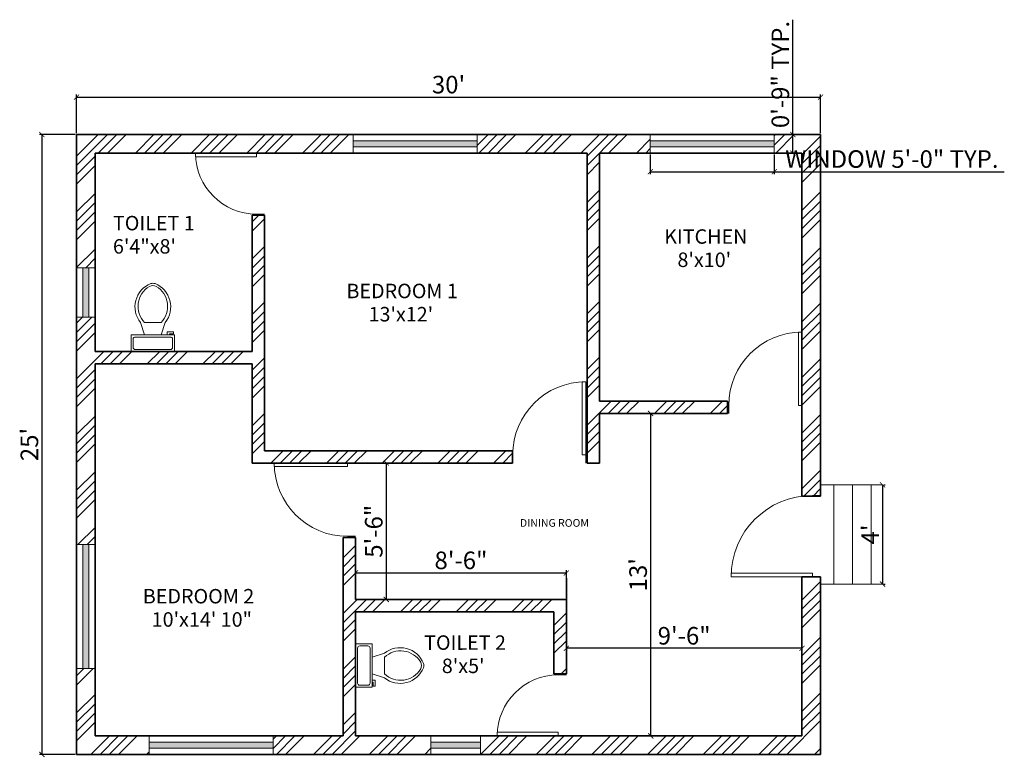
# Model space of a CAD drawing. Units: inches. Extents: x 3799 to 20199, y 1682 to 8087.
# Tile 24 of 30: x 16056 to 16532, y 2726 to 3083. Entities that reach past the tile are written whole.
import ezdxf

# ---------------------------------------------------------------- set-up
doc = ezdxf.new("R2010")
doc.units = ezdxf.units.IN
for name, color, linetype, lineweight in [('A-ANNO-DIMS', 2, 'Continuous', 18), ('A-AREA-IDEN', 7, 'Continuous', 18), ('A-DOOR', 3, 'Continuous', 18), ('A-FLOR-FIXT', 9, 'Continuous', 18), ('A-FLOR-STRS', 41, 'Continuous', 18), ('A-GLAZ', 152, 'Continuous', 18), ('A-GLAZ-PATT', 152, 'Continuous', 13), ('A-WALL', 7, 'Continuous', 35), ('A-WALL-PATT', 252, 'Continuous', 13)]:
    doc.layers.add(name, color=color, linetype=linetype, lineweight=lineweight)
doc.styles.get("Standard").update_dxf_attribs({"font": 'arial.ttf'})
doc.dimstyles.new('ISO-25', dxfattribs={"dimtxt": 8.5, "dimasz": 2.5, "dimexe": 1.25, "dimexo": 0.625, "dimtad": 1, "dimdec": 0, "dimlunit": 3, "dimtxsty": 'Standard', "dimblk": 'ARCHTICK', "dimcen": 2.5, "dimadec": 0, "dimazin": 0, "dimtfac": 1, "dimtdec": 0, "dimtmove": 0, "dimatfit": 3, "dimfxl": 1, "dimarcsym": 0})

# ---------------------------------------------------------------- blocks, each defined once
blk = doc.blocks.new('*U123')
for p, q in [((0, 0), (0, -100)), ((-900, 0), (-900, -100))]:
    blk.add_line(p, q)
blk.add_lwpolyline([(0, 0), (0, 900), (-43.75, 900), (-43.75, 0)], close=True)
blk.add_arc((0, 0), 900, 90, 180)
blk = doc.blocks.new('*U48')
for p, q in [((-750, 0), (-750, -100)), ((0, 0), (0, -100))]:
    blk.add_line(p, q)
blk.add_lwpolyline([(0, 0), (0, 750), (-43.75, 750), (-43.75, 0)], close=True)
blk.add_arc((0, 0), 750, 90, 180)
blk = doc.blocks.new('*U124')
for p, q in [((0, 0), (0, -100)), ((-900, 0), (-900, -100))]:
    blk.add_line(p, q)
blk.add_lwpolyline([(0, 0), (0, 900), (-43.75, 900), (-43.75, 0)], close=True)
blk.add_arc((0, 0), 900, 90, 180)
blk = doc.blocks.new('*U125')
for p, q in [((0, 0), (0, -100)), ((750, 0), (750, -100))]:
    blk.add_line(p, q)
blk.add_lwpolyline([(0, 0), (0, 750), (43.75, 750), (43.75, 0)], close=True)
blk.add_arc((0, 0), 750, 0, 90)
blk = doc.blocks.new('*U126')
for p, q in [((0, 0), (0, -100)), ((1000, 0), (1000, -100))]:
    blk.add_line(p, q)
blk.add_lwpolyline([(0, 0), (0, 1000), (43.75, 1000), (43.75, 0)], close=True)
blk.add_arc((0, 0), 1000, 0, 90)
blk = doc.blocks.new('_ArchTick')
at = {"color": 0, "linetype": 'ByBlock', "const_width": 0.15}
blk.add_lwpolyline([(-0.5, -0.5), (0.5, 0.5)], dxfattribs=at)
blk = doc.blocks.new('*D127')
at = {"layer": 'A-ANNO-DIMS', "color": 0, "lineweight": -2, "transparency": 16777216}
for p, q in [((16473.58, 2858.27), (16473.58, 2810.27)), ((16474.21, 2858.27), (16474.83, 2858.27)), ((16474.21, 2810.27), (16474.83, 2810.27))]:
    blk.add_line(p, q, dxfattribs=at)
at = {"layer": 'Defpoints', "color": 0, "transparency": 16777216}
for p in [(16473.58, 2858.27), (16473.58, 2810.27), (16473.58, 2810.27)]:
    blk.add_point(p, dxfattribs=at)
at = {"layer": 'A-ANNO-DIMS', "color": 0, "lineweight": -2, "transparency": 16777216, "xscale": 2.5, "yscale": 2.5, "zscale": 2.5}
for p, rotation in [((16473.58, 2858.27), 90), ((16473.58, 2810.27), 270)]:
    blk.add_blockref('_ArchTick', p, dxfattribs=dict(at, rotation=rotation))
at = {"layer": 'A-ANNO-DIMS', "color": 0, "transparency": 16777216, "insert": (16468.71, 2834.27), "char_height": 8.5, "attachment_point": 5, "rotation": 90}
blk.add_mtext("4'", dxfattribs=at)
blk = doc.blocks.new('*D128')
at = {"layer": 'A-ANNO-DIMS', "color": 0, "lineweight": -2, "transparency": 16777216}
for p, q in [((16293.96, 2868.83), (16232.22, 2868.83)), ((16233.47, 2868.83), (16233.47, 2802.83)), ((16293.96, 2802.83), (16232.22, 2802.83))]:
    blk.add_line(p, q, dxfattribs=at)
at = {"layer": 'Defpoints', "color": 0, "transparency": 16777216}
for p in [(16294.58, 2868.83), (16233.47, 2802.83), (16294.58, 2802.83)]:
    blk.add_point(p, dxfattribs=at)
at = {"layer": 'A-ANNO-DIMS', "color": 0, "lineweight": -2, "transparency": 16777216, "xscale": 2.5, "yscale": 2.5, "zscale": 2.5}
for p, rotation in [((16233.47, 2868.83), 90), ((16233.47, 2802.83), 270)]:
    blk.add_blockref('_ArchTick', p, dxfattribs=dict(at, rotation=rotation))
at = {"layer": 'A-ANNO-DIMS', "color": 0, "transparency": 16777216, "insert": (16228.5, 2835.83), "char_height": 8.5, "attachment_point": 5, "rotation": 90}
blk.add_mtext('5\'-6"', dxfattribs=at)
blk = doc.blocks.new('*D129')
at = {"layer": 'A-ANNO-DIMS', "color": 0, "lineweight": -2, "transparency": 16777216}
for p, q in [((16218.58, 2803.46), (16218.58, 2816.94)), ((16218.58, 2815.69), (16320.58, 2815.69)), ((16320.58, 2803.46), (16320.58, 2816.94))]:
    blk.add_line(p, q, dxfattribs=at)
at = {"layer": 'Defpoints', "color": 0, "transparency": 16777216}
for p in [(16320.58, 2815.69), (16218.58, 2802.83), (16320.58, 2802.83)]:
    blk.add_point(p, dxfattribs=at)
at = {"layer": 'A-ANNO-DIMS', "color": 0, "lineweight": -2, "transparency": 16777216, "xscale": 2.5, "yscale": 2.5, "zscale": 2.5, "rotation": 180}
blk.add_blockref('_ArchTick', (16218.58, 2815.69), dxfattribs=at)
at = {"layer": 'A-ANNO-DIMS', "color": 0, "lineweight": -2, "transparency": 16777216, "xscale": 2.5, "yscale": 2.5, "zscale": 2.5}
blk.add_blockref('_ArchTick', (16320.58, 2815.69), dxfattribs=at)
at = {"layer": 'A-ANNO-DIMS', "color": 0, "transparency": 16777216, "insert": (16269.58, 2820.66), "char_height": 8.5, "attachment_point": 5}
blk.add_mtext('8\'-6"', dxfattribs=at)
blk = doc.blocks.new('*D130')
at = {"layer": 'A-ANNO-DIMS', "color": 0, "lineweight": -2, "transparency": 16777216}
for p, q in [((16337.21, 2892.83), (16362.62, 2892.83)), ((16361.37, 2892.83), (16361.37, 2736.83)), ((16337.21, 2736.83), (16362.62, 2736.83))]:
    blk.add_line(p, q, dxfattribs=at)
at = {"layer": 'Defpoints', "color": 0, "transparency": 16777216}
for p in [(16336.58, 2892.83), (16336.58, 2736.83), (16361.37, 2736.83)]:
    blk.add_point(p, dxfattribs=at)
at = {"layer": 'A-ANNO-DIMS', "color": 0, "lineweight": -2, "transparency": 16777216, "xscale": 2.5, "yscale": 2.5, "zscale": 2.5}
for p, rotation in [((16361.37, 2892.83), 90), ((16361.37, 2736.83), 270)]:
    blk.add_blockref('_ArchTick', p, dxfattribs=dict(at, rotation=rotation))
at = {"layer": 'A-ANNO-DIMS', "color": 0, "transparency": 16777216, "insert": (16356.4, 2814.83), "char_height": 8.5, "attachment_point": 5, "rotation": 90}
blk.add_mtext("13'", dxfattribs=at)
blk = doc.blocks.new('*D131')
at = {"layer": 'A-ANNO-DIMS', "color": 0, "lineweight": -2, "transparency": 16777216}
for p, q in [((16320.58, 2813.18), (16320.58, 2777.94)), ((16434.58, 2813.18), (16434.58, 2777.94)), ((16434.58, 2779.19), (16320.58, 2779.19))]:
    blk.add_line(p, q, dxfattribs=at)
at = {"layer": 'Defpoints', "color": 0, "transparency": 16777216}
for p in [(16320.58, 2813.8), (16434.58, 2813.8), (16320.58, 2779.19)]:
    blk.add_point(p, dxfattribs=at)
at = {"layer": 'A-ANNO-DIMS', "color": 0, "lineweight": -2, "transparency": 16777216, "xscale": 2.5, "yscale": 2.5, "zscale": 2.5, "rotation": 180}
blk.add_blockref('_ArchTick', (16320.58, 2779.19), dxfattribs=at)
at = {"layer": 'A-ANNO-DIMS', "color": 0, "lineweight": -2, "transparency": 16777216, "xscale": 2.5, "yscale": 2.5, "zscale": 2.5}
blk.add_blockref('_ArchTick', (16434.58, 2779.19), dxfattribs=at)
at = {"layer": 'A-ANNO-DIMS', "color": 0, "transparency": 16777216, "insert": (16377.58, 2784.16), "char_height": 8.5, "attachment_point": 5}
blk.add_mtext('9\'-6"', dxfattribs=at)
blk = doc.blocks.new('*D132')
at = {"layer": 'A-ANNO-DIMS', "color": 0, "lineweight": -2, "transparency": 16777216}
for p, q in [((16083.58, 3028.46), (16083.58, 3047.16)), ((16083.58, 3045.91), (16443.58, 3045.91)), ((16443.58, 3028.46), (16443.58, 3047.16))]:
    blk.add_line(p, q, dxfattribs=at)
at = {"layer": 'Defpoints', "color": 0, "transparency": 16777216}
for p in [(16443.58, 3045.91), (16083.58, 3027.83), (16443.58, 3027.83)]:
    blk.add_point(p, dxfattribs=at)
at = {"layer": 'A-ANNO-DIMS', "color": 0, "lineweight": -2, "transparency": 16777216, "xscale": 2.5, "yscale": 2.5, "zscale": 2.5, "rotation": 180}
blk.add_blockref('_ArchTick', (16083.58, 3045.91), dxfattribs=at)
at = {"layer": 'A-ANNO-DIMS', "color": 0, "lineweight": -2, "transparency": 16777216, "xscale": 2.5, "yscale": 2.5, "zscale": 2.5}
blk.add_blockref('_ArchTick', (16443.58, 3045.91), dxfattribs=at)
at = {"layer": 'A-ANNO-DIMS', "color": 0, "transparency": 16777216, "insert": (16263.58, 3050.88), "char_height": 8.5, "attachment_point": 5}
blk.add_mtext("30'", dxfattribs=at)
blk = doc.blocks.new('*D133')
at = {"layer": 'A-ANNO-DIMS', "color": 0, "lineweight": -2, "transparency": 16777216}
for p, q in [((16082.96, 3027.83), (16065.58, 3027.83)), ((16066.83, 3027.83), (16066.83, 2727.83)), ((16082.96, 2727.83), (16065.58, 2727.83))]:
    blk.add_line(p, q, dxfattribs=at)
at = {"layer": 'Defpoints', "color": 0, "transparency": 16777216}
for p in [(16083.58, 3027.83), (16066.83, 2727.83), (16083.58, 2727.83)]:
    blk.add_point(p, dxfattribs=at)
at = {"layer": 'A-ANNO-DIMS', "color": 0, "lineweight": -2, "transparency": 16777216, "xscale": 2.5, "yscale": 2.5, "zscale": 2.5}
for p, rotation in [((16066.83, 3027.83), 90), ((16066.83, 2727.83), 270)]:
    blk.add_blockref('_ArchTick', p, dxfattribs=dict(at, rotation=rotation))
at = {"layer": 'A-ANNO-DIMS', "color": 0, "transparency": 16777216, "insert": (16061.87, 2877.83), "char_height": 8.5, "attachment_point": 5, "rotation": 90}
blk.add_mtext("25'", dxfattribs=at)
blk = doc.blocks.new('Toilet - top')
for p, q in [((9.5, -6), (9.5, -2)), ((-10, -8.5), (-8, -8.5)), ((-10, -9.5), (-10, -8.5)), ((-7, -9.5), (-10, -9.5)), ((-8, -8.5), (-8, -8)), ((-7, -8), (-7, -9.5)), ((-4, -8), (-6, -14)), ((4, -8), (6, -14)), ((4, -14), (-4, -14))]:
    blk.add_line(p, q)
blk.add_lwpolyline([(10.5, -8), (10.5, 0), (-10.5, 0), (-10.5, -8)], close=True)
for points in [[(-9.5, -2), (-9.5, -6)], [(8.5, -1), (-8.5, -1)], [(-8.5, -7), (8.5, -7)]]:
    blk.add_lwpolyline(points)
for centre, radius, start, end in [((-8.62, -1.88), 0.884, 81.8699, 188.1301), ((8.62, -1.88), 0.884, 351.8699, 98.1301), ((-8.62, -6.12), 0.884, 171.8699, 278.1301), ((8.62, -6.12), 0.884, 261.8699, 8.1301), ((3.52, -21.58), 12.17, 141.4691, 247.9714), ((4.2, -21.82), 11.33, 136.3677, 238.9468), ((-3.52, -21.58), 12.17, 292.0284, 38.5307), ((-4.2, -21.82), 11.33, 301.053, 43.6321), ((0, -27.88), 4, 245.7318, 294.2682), ((0, -29), 4, 254.8605, 285.1395)]:
    blk.add_arc(centre, radius, start, end)
blk = doc.blocks.new('WIN-24IN-9IN-FRAME')
for p, q in [((0, 24), (9, 24)), ((3, 0), (3, 24)), ((6, 0), (6, 24)), ((0, 0), (9, 0))]:
    blk.add_line(p, q)
blk = doc.blocks.new('WIN-60IN-9IN-FRAME')
for p, q in [((0, 9), (0, 0)), ((60, 6), (0, 6)), ((60, 9), (60, 0)), ((60, 3), (0, 3))]:
    blk.add_line(p, q)
blk = doc.blocks.new('*D244')
at = {"layer": 'A-ANNO-DIMS', "color": 0, "lineweight": -2, "transparency": 16777216}
for p, q in [((16361.18, 3018.21), (16361.18, 3008.58)), ((16421.18, 3018.21), (16421.18, 3008.58)), ((16361.18, 3009.83), (16421.18, 3009.83)), ((16421.18, 3009.83), (16532.49, 3009.83))]:
    blk.add_line(p, q, dxfattribs=at)
at = {"layer": 'Defpoints', "color": 0, "transparency": 16777216}
for p in [(16361.18, 3018.83), (16421.18, 3018.83), (16421.18, 3009.83)]:
    blk.add_point(p, dxfattribs=at)
at = {"layer": 'A-ANNO-DIMS', "color": 0, "lineweight": -2, "transparency": 16777216, "xscale": 2.5, "yscale": 2.5, "zscale": 2.5, "rotation": 180}
blk.add_blockref('_ArchTick', (16361.18, 3009.83), dxfattribs=at)
at = {"layer": 'A-ANNO-DIMS', "color": 0, "lineweight": -2, "transparency": 16777216, "xscale": 2.5, "yscale": 2.5, "zscale": 2.5}
blk.add_blockref('_ArchTick', (16421.18, 3009.83), dxfattribs=at)
at = {"layer": 'A-ANNO-DIMS', "color": 0, "transparency": 16777216, "insert": (16478.08, 3014.86), "char_height": 8.5, "attachment_point": 5}
blk.add_mtext('WINDOW 5\'-0" TYP.', dxfattribs=at)
blk = doc.blocks.new('*D245')
at = {"layer": 'A-ANNO-DIMS', "color": 0, "lineweight": -2, "transparency": 16777216}
for p, q in [((16430.18, 3027.83), (16430.18, 3083.4)), ((16421.8, 3027.83), (16431.43, 3027.83)), ((16430.18, 3018.83), (16430.18, 3027.83)), ((16421.8, 3018.83), (16431.43, 3018.83))]:
    blk.add_line(p, q, dxfattribs=at)
at = {"layer": 'Defpoints', "color": 0, "transparency": 16777216}
for p in [(16421.18, 3027.83), (16430.18, 3027.83), (16421.18, 3018.83)]:
    blk.add_point(p, dxfattribs=at)
at = {"layer": 'A-ANNO-DIMS', "color": 0, "lineweight": -2, "transparency": 16777216, "xscale": 2.5, "yscale": 2.5, "zscale": 2.5}
for p, rotation in [((16430.18, 3027.83), 90), ((16430.18, 3018.83), 270)]:
    blk.add_blockref('_ArchTick', p, dxfattribs=dict(at, rotation=rotation))
at = {"layer": 'A-ANNO-DIMS', "color": 0, "transparency": 16777216, "insert": (16425.21, 3056.86), "char_height": 8.5, "attachment_point": 5, "rotation": 90}
blk.add_mtext('0\'-9" TYP.', dxfattribs=at)

msp = doc.modelspace()

# ---------------------------------------------------------------- hatches: boundary and pattern name
at = {"layer": 'A-GLAZ-PATT'}
h = msp.add_hatch(color=256, dxfattribs=at)
h.dxf.hatch_style = 1
h.set_gradient(color1=(0, 0, 255), color2=(122, 175, 223), name='SPHERICAL')
h.paths.add_polyline_path([(16421.18, 3024.83), (16361.18, 3024.83), (16361.18, 3021.83), (16421.18, 3021.83)])
h.paths.add_polyline_path([(16277.44, 3024.83), (16217.44, 3024.83), (16217.44, 3021.83), (16277.44, 3021.83)])
h.paths.add_polyline_path([(16089.58, 2963.38), (16086.58, 2963.38), (16086.58, 2939.38), (16089.58, 2939.38)])
h.paths.add_polyline_path([(16089.58, 2829.38), (16086.58, 2829.38), (16086.58, 2769.38), (16089.58, 2769.38)])
h.paths.add_polyline_path([(16178.71, 2733.83), (16118.71, 2733.83), (16118.71, 2730.83), (16178.71, 2730.83)])
h.paths.add_polyline_path([(16279.08, 2733.83), (16255.08, 2733.83), (16255.08, 2730.83), (16279.08, 2730.83)])
at = {"layer": 'A-WALL-PATT'}
h = msp.add_hatch(dxfattribs=at)
h.set_pattern_fill('ANSI34', color=256)
h.paths.add_polyline_path([(16118.71, 2736.83), (16092.58, 2736.83), (16092.58, 2769.38), (16083.58, 2769.38), (16083.58, 2727.83), (16118.71, 2727.83)])
h.paths.add_polyline_path([(16255.08, 2736.83), (16218.58, 2736.83), (16218.58, 2796.83), (16314.58, 2796.83), (16314.58, 2766.83), (16320.58, 2766.83), (16320.58, 2802.83), (16218.58, 2802.83), (16218.58, 2832.83), (16212.58, 2832.83), (16212.58, 2736.83), (16178.71, 2736.83), (16178.71, 2727.83), (16255.08, 2727.83)])
h.paths.add_polyline_path([(16443.58, 2813.8), (16434.58, 2813.8), (16434.58, 2736.83), (16320.58, 2736.83), (16279.08, 2736.83), (16279.08, 2727.83), (16443.58, 2727.83)])
h.paths.add_polyline_path([(16443.58, 3027.83), (16421.18, 3027.83), (16421.18, 3018.83), (16434.58, 3018.83), (16434.58, 2892.83), (16434.58, 2852.8), (16443.58, 2852.8)])
h.paths.add_polyline_path([(16398.58, 2898.83), (16336.58, 2898.83), (16336.58, 3018.83), (16361.18, 3018.83), (16361.18, 3027.83), (16277.44, 3027.83), (16277.44, 3018.83), (16330.58, 3018.83), (16330.58, 2868.83), (16336.58, 2868.83), (16336.58, 2892.83), (16398.58, 2892.83)])
h.paths.add_polyline_path([(16294.58, 2874.83), (16174.58, 2874.83), (16174.58, 2988.83), (16168.58, 2988.83), (16168.58, 2922.83), (16092.58, 2922.83), (16092.58, 2939.38), (16083.58, 2939.38), (16083.58, 2829.38), (16092.58, 2829.38), (16092.58, 2916.83), (16168.58, 2916.83), (16168.58, 2868.83), (16294.58, 2868.83)])
h.paths.add_polyline_path([(16092.58, 3018.83), (16174.58, 3018.83), (16217.44, 3018.83), (16217.44, 3027.83), (16083.58, 3027.83), (16083.58, 2963.38), (16092.58, 2963.38)])

# ---------------------------------------------------------------- linework, layer by layer
at = {"layer": 'A-FLOR-STRS'}
for p, q in [((16443.58, 2858.27), (16473.58, 2858.27)), ((16450.02, 2858.27), (16450.02, 2810.27)), ((16459.02, 2858.27), (16459.02, 2810.27)), ((16468.02, 2858.27), (16468.02, 2810.27)), ((16443.58, 2810.27), (16473.58, 2810.27))]:
    msp.add_line(p, q, dxfattribs=at)
at = {"layer": 'A-WALL'}
for p, q in [((16443.58, 3027.83), (16083.58, 3027.83)), ((16083.58, 3027.83), (16083.58, 2727.83)), ((16443.58, 2852.8), (16443.58, 3027.83)), ((16092.58, 3018.83), (16092.58, 2922.83)), ((16174.58, 3018.83), (16092.58, 3018.83)), ((16330.58, 3018.83), (16174.58, 3018.83)), ((16330.58, 3018.83), (16330.58, 2868.83)), ((16434.58, 3018.83), (16336.58, 3018.83)), ((16336.58, 3018.83), (16336.58, 2898.83)), ((16336.58, 3018.83), (16336.58, 2898.83)), ((16434.58, 2892.83), (16434.58, 3018.83)), ((16168.58, 2988.83), (16168.58, 2922.83)), ((16174.58, 2988.83), (16168.58, 2988.83)), ((16174.58, 2988.83), (16174.58, 2874.83)), ((16168.58, 2922.83), (16092.58, 2922.83)), ((16168.58, 2916.83), (16092.58, 2916.83)), ((16092.58, 2916.83), (16092.58, 2736.83)), ((16168.58, 2916.83), (16168.58, 2868.83)), ((16398.58, 2898.83), (16336.58, 2898.83)), ((16398.58, 2892.83), (16398.58, 2898.83)), ((16398.58, 2892.83), (16336.58, 2892.83)), ((16336.58, 2892.83), (16336.58, 2868.83)), ((16434.58, 2852.8), (16434.58, 2892.83)), ((16294.58, 2874.83), (16174.58, 2874.83)), ((16294.58, 2874.83), (16294.58, 2868.83)), ((16294.58, 2868.83), (16168.58, 2868.83)), ((16336.58, 2868.83), (16330.58, 2868.83)), ((16434.58, 2852.8), (16443.58, 2852.8)), ((16212.58, 2832.83), (16212.58, 2736.83)), ((16218.58, 2832.83), (16212.58, 2832.83)), ((16218.58, 2832.83), (16218.58, 2802.83)), ((16434.58, 2736.83), (16434.58, 2813.8)), ((16434.58, 2813.8), (16443.58, 2813.8)), ((16443.58, 2727.83), (16443.58, 2813.8)), ((16218.58, 2802.83), (16320.58, 2802.83)), ((16320.58, 2802.83), (16320.58, 2766.83)), ((16218.58, 2796.83), (16314.58, 2796.83)), ((16218.58, 2796.83), (16218.58, 2736.83)), ((16314.58, 2796.83), (16314.58, 2766.83)), ((16314.58, 2766.83), (16320.58, 2766.83)), ((16092.58, 2736.83), (16212.58, 2736.83)), ((16218.58, 2736.83), (16320.58, 2736.83)), ((16320.58, 2736.83), (16434.58, 2736.83)), ((16083.58, 2727.83), (16443.58, 2727.83))]:
    msp.add_line(p, q, dxfattribs=at)

# ---------------------------------------------------------------- block references
at = {"layer": 'A-DOOR', "xscale": 0.0393700787401575, "yscale": 0.0393700787401575, "zscale": 0.0393700787401575, "rotation": 90.00000000000003}
for name, p in [('*U48', (16170.65, 3018.83)), ('*U124', (16214.65, 2868.83)), ('*U126', (16439.65, 2813.8)), ('*U125', (16316.65, 2736.83))]:
    msp.add_blockref(name, p, dxfattribs=at)
at = {"layer": 'A-DOOR', "xscale": 0.0393700787401575, "yscale": 0.0393700787401575, "zscale": 0.0393700787401575}
for p in [(16434.58, 2896.77), (16330.02, 2872.77)]:
    msp.add_blockref('*U123', p, dxfattribs=at)
at = {"layer": 'A-FLOR-FIXT'}
for p, rotation in [((16120.5, 2922.83), 180), ((16218.58, 2770.85), 90)]:
    msp.add_blockref('Toilet - top', p, dxfattribs=dict(at, rotation=rotation))
at = {"layer": 'A-GLAZ'}
for name, p in [('WIN-60IN-9IN-FRAME', (16217.44, 3018.83)), ('WIN-60IN-9IN-FRAME', (16361.18, 3018.83)), ('WIN-24IN-9IN-FRAME', (16083.58, 2939.38)), ('WIN-60IN-9IN-FRAME', (16118.71, 2727.83))]:
    msp.add_blockref(name, p, dxfattribs=at)
at = {"layer": 'A-GLAZ', "rotation": 90}
for name, p in [('WIN-60IN-9IN-FRAME', (16092.58, 2769.38)), ('WIN-24IN-9IN-FRAME', (16279.08, 2727.83))]:
    msp.add_blockref(name, p, dxfattribs=at)

# ---------------------------------------------------------------- texts
at = {"layer": 'A-AREA-IDEN'}
for s, height, p in [('TOILET 1', 7, (16101.19, 2981.46)), ('6\'4"x8\'', 7, (16101.19, 2970.21)), ('KITCHEN', 7, (16367.93, 2974.96)), ("   8'x10'", 7, (16367.93, 2963.71)), ('BEDROOM 1', 7, (16214.18, 2948.62)), ("     13'x12'", 7, (16214.18, 2937.38)), ('DINING ROOM', 3.7275, (16298.11, 2838.01)), ('BEDROOM 2', 7, (16115.66, 2800.91)), ('  10\'x14\' 10"', 7, (16115.66, 2789.66)), ('TOILET 2', 7, (16251.77, 2778.46)), ("    8'x5'", 7, (16251.77, 2767.21))]:
    msp.add_text(s, height=height, rotation=0.0019, dxfattribs=at).set_placement(p)

# ---------------------------------------------------------------- dimensions: what is measured, and where the dimension line sits
at = {"layer": 'A-ANNO-DIMS'}
dim = msp.add_linear_dim(base=(16430.18, 3027.83), p1=(16421.18, 3018.83), p2=(16421.18, 3027.83), angle=90, text='<> TYP.', dimstyle='ISO-25', override={"dimdec": 1, "dimlfac": 1, "dimrnd": 0, "dimzin": 1, "dimdsep": 46, "dimlunit": 4, "dimfrac": 2}, dxfattribs=at)
dim.commit()
dim.dimension.update_dxf_attribs({"geometry": '*D245', "text_midpoint": (16425.21, 3056.86)})
for base, p1, p2, picture, middle in [((16443.58, 3045.91), (16083.58, 3027.83), (16443.58, 3027.83), '*D132', (16263.58, 3050.88)), ((16320.58, 2815.69), (16218.58, 2802.83), (16320.58, 2802.83), '*D129', (16269.58, 2820.66)), ((16320.58, 2779.19), (16434.58, 2813.8), (16320.58, 2813.8), '*D131', (16377.58, 2784.16))]:
    dim = msp.add_linear_dim(base=base, p1=p1, p2=p2, dimstyle='ISO-25', override={"dimclrd": 0, "dimclre": 0, "dimclrt": 0}, dxfattribs=at)
    dim.commit()
    dim.dimension.update_dxf_attribs({"geometry": picture, "text_midpoint": middle})
dim = msp.add_linear_dim(base=(16421.18, 3009.83), p1=(16361.18, 3018.83), p2=(16421.18, 3018.83), text='WINDOW <> TYP.', dimstyle='ISO-25', override={"dimdec": 1, "dimlfac": 1, "dimrnd": 0, "dimzin": 1, "dimdsep": 46, "dimlunit": 4, "dimfrac": 2}, dxfattribs=at)
dim.commit()
dim.dimension.update_dxf_attribs({"geometry": '*D244', "text_midpoint": (16478.08, 3014.86)})
for base, p1, p2, picture, middle in [((16066.83, 2727.83), (16083.58, 3027.83), (16083.58, 2727.83), '*D133', (16061.87, 2877.83)), ((16361.37, 2736.83), (16336.58, 2892.83), (16336.58, 2736.83), '*D130', (16356.4, 2814.83)), ((16233.47, 2802.83), (16294.58, 2868.83), (16294.58, 2802.83), '*D128', (16228.5, 2835.83)), ((16473.58, 2810.27), (16473.58, 2858.27), (16473.58, 2810.27), '*D127', (16468.71, 2834.27))]:
    dim = msp.add_linear_dim(base=base, p1=p1, p2=p2, angle=90, dimstyle='ISO-25', override={"dimclrd": 0, "dimclre": 0, "dimclrt": 0}, dxfattribs=at)
    dim.commit()
    dim.dimension.update_dxf_attribs({"geometry": picture, "text_midpoint": middle})

doc.saveas('drawing.dxf')
